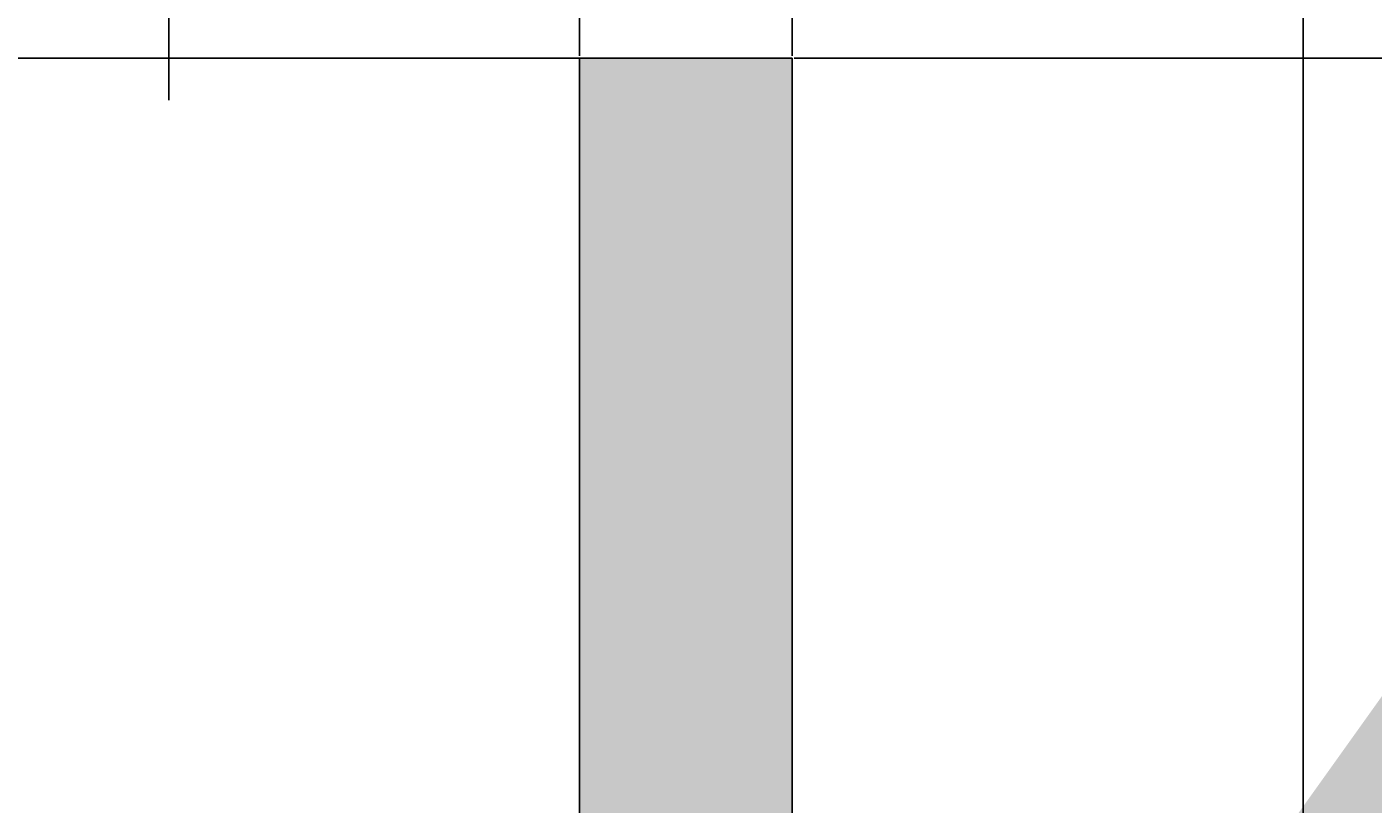
# Model space of a CAD drawing. Units: millimetres. Extents: x -22994 to 29398, y -19990 to 20176.
# Tile 112 of 135: x 166 to 204, y 155 to 177. Entities that reach past the tile are written whole.
import ezdxf

# ---------------------------------------------------------------- set-up
doc = ezdxf.new("R2010")
doc.units = ezdxf.units.MM
doc.header["$MEASUREMENT"] = 0
for name, color, linetype, lineweight in [('M-ANNO-SYMB', 7, 'Continuous', 25), ('M-DIMS', 2, 'Continuous', 18), ('M-EQPM', 7, 'Continuous', 25), ('M-EQPM-PATT', 7, 'Continuous', 18)]:
    doc.layers.add(name, color=color, linetype=linetype, lineweight=lineweight)
doc.styles.get("Standard").update_dxf_attribs({"font": 'arial.ttf'})
doc.dimstyles.get("Standard").update_dxf_attribs({"dimtxt": 0.18, "dimasz": 10000, "dimexe": 0.18, "dimexo": 0.0625, "dimgap": 0.09, "dimtad": 0, "dimtih": 1, "dimtoh": 1, "dimdec": 0, "dimzin": 0, "dimdsep": 46, "dimtxsty": 'Standard', "dimcen": 0.09, "dimadec": 0, "dimazin": 0, "dimtfac": 1, "dimtdec": 0, "dimtofl": 0, "dimtmove": 0, "dimatfit": 3, "dimfxl": 1, "dimtolj": 1, "dimtzin": 0, "dimlwd": 30, "dimarcsym": 0})

# ---------------------------------------------------------------- blocks, each defined once
blk = doc.blocks.new('*D2')
at = {"layer": 'Defpoints', "color": 0, "transparency": 16777216}
for p in [(6.677, 10.271), (290.852, 10.271), (290.852, -5.079)]:
    blk.add_point(p, dxfattribs=at)
at = {"layer": 'M-DIMS', "color": 0, "lineweight": -2, "transparency": 16777216}
for p, q in [((6.677, 10.209), (6.677, -5.259)), ((290.852, 10.209), (290.852, -5.259))]:
    blk.add_line(p, q, dxfattribs=at)
at = {"layer": 'M-DIMS', "color": 0, "lineweight": 30, "transparency": 16777216}
for p, q in [((-9993.323, -5.079), (-19993.323, -5.079)), ((10290.852, -5.079), (20290.852, -5.079))]:
    blk.add_line(p, q, dxfattribs=at)
at = {"layer": 'M-DIMS', "color": 0, "transparency": 16777216}
for points in [[(-9993.323, 1661.588), (-9993.323, -1671.745), (6.677, -5.079)], [(10290.852, 1661.588), (10290.852, -1671.745), (290.852, -5.079)]]:
    blk.add_solid(points, dxfattribs=at)
at = {"layer": 'M-DIMS', "color": 0, "transparency": 16777216, "insert": (148.765, -5.079), "char_height": 0.18, "attachment_point": 5}
blk.add_mtext('\\A1;284.2', dxfattribs=at)
blk = doc.blocks.new('*D3')
at = {"layer": 'Defpoints', "color": 0, "transparency": 16777216}
for p in [(110.265, 204.165), (110.265, 176.366), (95.833, 127.967)]:
    blk.add_point(p, dxfattribs=at)
at = {"layer": 'M-DIMS', "color": 0, "lineweight": 30, "transparency": 16777216}
for p, q in [((-9904.167, 204.165), (-19904.167, 204.165)), ((10110.265, 204.165), (20110.265, 204.165))]:
    blk.add_line(p, q, dxfattribs=at)
at = {"layer": 'M-DIMS', "color": 0, "lineweight": -2, "transparency": 16777216}
for p, q in [((95.833, 128.03), (95.833, 204.345)), ((110.265, 176.429), (110.265, 204.345))]:
    blk.add_line(p, q, dxfattribs=at)
at = {"layer": 'M-DIMS', "color": 0, "transparency": 16777216}
for points in [[(-9904.167, 1870.832), (-9904.167, -1462.501), (95.833, 204.165)], [(10110.265, 1870.832), (10110.265, -1462.501), (110.265, 204.165)]]:
    blk.add_solid(points, dxfattribs=at)
at = {"layer": 'M-DIMS', "color": 0, "transparency": 16777216, "insert": (103.049, 204.165), "char_height": 0.18, "attachment_point": 5}
blk.add_mtext('\\A1;14.432', dxfattribs=at)
blk = doc.blocks.new('*D4')
at = {"layer": 'Defpoints', "color": 0, "transparency": 16777216}
for p in [(116.265, 204.165), (110.265, 176.366), (116.265, 176.366)]:
    blk.add_point(p, dxfattribs=at)
at = {"layer": 'M-DIMS', "color": 0, "lineweight": 30, "transparency": 16777216}
for p, q in [((-9889.735, 204.165), (-19889.735, 204.165)), ((10116.265, 204.165), (20116.265, 204.165))]:
    blk.add_line(p, q, dxfattribs=at)
at = {"layer": 'M-DIMS', "color": 0, "lineweight": -2, "transparency": 16777216}
for p, q in [((110.265, 176.429), (110.265, 204.345)), ((116.265, 176.429), (116.265, 204.345))]:
    blk.add_line(p, q, dxfattribs=at)
at = {"layer": 'M-DIMS', "color": 0, "transparency": 16777216}
for points in [[(-9889.735, 1870.832), (-9889.735, -1462.501), (110.265, 204.165)], [(10116.265, 1870.832), (10116.265, -1462.501), (116.265, 204.165)]]:
    blk.add_solid(points, dxfattribs=at)
at = {"layer": 'M-DIMS', "color": 0, "transparency": 16777216, "insert": (113.265, 204.165), "char_height": 0.18, "attachment_point": 5}
blk.add_mtext('\\A1;6', dxfattribs=at)
blk = doc.blocks.new('*D5')
at = {"layer": 'Defpoints', "color": 0, "transparency": 16777216}
for p in [(181.265, 204.165), (116.265, 176.366), (181.265, 176.366)]:
    blk.add_point(p, dxfattribs=at)
at = {"layer": 'M-DIMS', "color": 0, "lineweight": 30, "transparency": 16777216}
for p, q in [((-9883.735, 204.165), (-19883.735, 204.165)), ((10181.265, 204.165), (20181.265, 204.165))]:
    blk.add_line(p, q, dxfattribs=at)
at = {"layer": 'M-DIMS', "color": 0, "lineweight": -2, "transparency": 16777216}
for p, q in [((116.265, 176.429), (116.265, 204.345)), ((181.265, 176.429), (181.265, 204.345))]:
    blk.add_line(p, q, dxfattribs=at)
at = {"layer": 'M-DIMS', "color": 0, "transparency": 16777216}
for points in [[(-9883.735, 1870.832), (-9883.735, -1462.501), (116.265, 204.165)], [(10181.265, 1870.832), (10181.265, -1462.501), (181.265, 204.165)]]:
    blk.add_solid(points, dxfattribs=at)
at = {"layer": 'M-DIMS', "color": 0, "transparency": 16777216, "insert": (148.765, 204.165), "char_height": 0.18, "attachment_point": 5}
blk.add_mtext('\\A1;65', dxfattribs=at)
blk = doc.blocks.new('*D6')
at = {"layer": 'Defpoints', "color": 0, "transparency": 16777216}
for p in [(187.265, 204.165), (181.265, 176.366), (187.265, 176.366)]:
    blk.add_point(p, dxfattribs=at)
at = {"layer": 'M-DIMS', "color": 0, "lineweight": 30, "transparency": 16777216}
for p, q in [((-9818.735, 204.165), (-19818.735, 204.165)), ((10187.265, 204.165), (20187.265, 204.165))]:
    blk.add_line(p, q, dxfattribs=at)
at = {"layer": 'M-DIMS', "color": 0, "lineweight": -2, "transparency": 16777216}
for p, q in [((181.265, 176.429), (181.265, 204.345)), ((187.265, 176.429), (187.265, 204.345))]:
    blk.add_line(p, q, dxfattribs=at)
at = {"layer": 'M-DIMS', "color": 0, "transparency": 16777216}
for points in [[(-9818.735, 1870.832), (-9818.735, -1462.501), (181.265, 204.165)], [(10187.265, 1870.832), (10187.265, -1462.501), (187.265, 204.165)]]:
    blk.add_solid(points, dxfattribs=at)
at = {"layer": 'M-DIMS', "color": 0, "transparency": 16777216, "insert": (184.265, 204.165), "char_height": 0.18, "attachment_point": 5}
blk.add_mtext('\\A1;6', dxfattribs=at)
blk = doc.blocks.new('*D7')
at = {"layer": 'Defpoints', "color": 0, "transparency": 16777216}
for p in [(201.697, 204.165), (187.265, 176.366), (201.697, 127.967)]:
    blk.add_point(p, dxfattribs=at)
at = {"layer": 'M-DIMS', "color": 0, "lineweight": 30, "transparency": 16777216}
for p, q in [((-9812.735, 204.165), (-19812.735, 204.165)), ((10201.697, 204.165), (20201.697, 204.165))]:
    blk.add_line(p, q, dxfattribs=at)
at = {"layer": 'M-DIMS', "color": 0, "lineweight": -2, "transparency": 16777216}
for p, q in [((187.265, 176.429), (187.265, 204.345)), ((201.697, 128.03), (201.697, 204.345))]:
    blk.add_line(p, q, dxfattribs=at)
at = {"layer": 'M-DIMS', "color": 0, "transparency": 16777216}
for points in [[(-9812.735, 1870.832), (-9812.735, -1462.501), (187.265, 204.165)], [(10201.697, 1870.832), (10201.697, -1462.501), (201.697, 204.165)]]:
    blk.add_solid(points, dxfattribs=at)
at = {"layer": 'M-DIMS', "color": 0, "transparency": 16777216, "insert": (194.481, 204.165), "char_height": 0.18, "attachment_point": 5}
blk.add_mtext('\\A1;14.432', dxfattribs=at)
blk = doc.blocks.new('*D8')
at = {"layer": 'Defpoints', "color": 0, "transparency": 16777216}
for p in [(227.648, 204.165), (227.648, 146.73), (201.697, 127.967)]:
    blk.add_point(p, dxfattribs=at)
at = {"layer": 'M-DIMS', "color": 0, "lineweight": 30, "transparency": 16777216}
for p, q in [((-9798.303, 204.165), (-19798.303, 204.165)), ((10227.648, 204.165), (20227.648, 204.165))]:
    blk.add_line(p, q, dxfattribs=at)
at = {"layer": 'M-DIMS', "color": 0, "lineweight": -2, "transparency": 16777216}
for p, q in [((201.697, 128.03), (201.697, 204.345)), ((227.648, 146.792), (227.648, 204.345))]:
    blk.add_line(p, q, dxfattribs=at)
at = {"layer": 'M-DIMS', "color": 0, "transparency": 16777216}
for points in [[(-9798.303, 1870.832), (-9798.303, -1462.501), (201.697, 204.165)], [(10227.648, 1870.832), (10227.648, -1462.501), (227.648, 204.165)]]:
    blk.add_solid(points, dxfattribs=at)
at = {"layer": 'M-DIMS', "color": 0, "transparency": 16777216, "insert": (214.673, 204.165), "char_height": 0.18, "attachment_point": 5}
blk.add_mtext('\\A1;25.95', dxfattribs=at)
blk = doc.blocks.new('*D9')
at = {"layer": 'Defpoints', "color": 0, "transparency": 16777216}
for p in [(187.265, 176.366), (306.202, 176.366), (290.852, 10.271)]:
    blk.add_point(p, dxfattribs=at)
at = {"layer": 'M-DIMS', "color": 0, "lineweight": 30, "transparency": 16777216}
for p, q in [((306.202, 10176.366), (306.202, 20176.366)), ((306.202, -9989.729), (306.202, -19989.729))]:
    blk.add_line(p, q, dxfattribs=at)
at = {"layer": 'M-DIMS', "color": 0, "lineweight": -2, "transparency": 16777216}
for p, q in [((187.327, 176.366), (306.382, 176.366)), ((290.915, 10.271), (306.382, 10.271))]:
    blk.add_line(p, q, dxfattribs=at)
at = {"layer": 'M-DIMS', "color": 0, "transparency": 16777216}
for points in [[(-1360.465, 10176.366), (1972.869, 10176.366), (306.202, 176.366)], [(-1360.465, -9989.729), (1972.869, -9989.729), (306.202, 10.271)]]:
    blk.add_solid(points, dxfattribs=at)
at = {"layer": 'M-DIMS', "color": 0, "transparency": 16777216, "insert": (306.202, 93.319), "char_height": 0.18, "attachment_point": 5}
blk.add_mtext('\\A1;166.1', dxfattribs=at)
blk = doc.blocks.new('*D10')
at = {"layer": 'Defpoints', "color": 0, "transparency": 16777216}
for p in [(125.65, 136.071), (133.346, 136.071), (133.346, -5.079)]:
    blk.add_point(p, dxfattribs=at)
at = {"layer": 'M-DIMS', "color": 0, "lineweight": -2, "transparency": 16777216}
for p, q in [((125.65, 136.009), (125.65, -5.259)), ((133.346, 136.009), (133.346, -5.259))]:
    blk.add_line(p, q, dxfattribs=at)
at = {"layer": 'M-DIMS', "color": 0, "lineweight": 30, "transparency": 16777216}
for p, q in [((-9874.35, -5.079), (-19874.35, -5.079)), ((10133.346, -5.079), (20133.346, -5.079))]:
    blk.add_line(p, q, dxfattribs=at)
at = {"layer": 'M-DIMS', "color": 0, "transparency": 16777216}
for points in [[(-9874.35, 1661.588), (-9874.35, -1671.745), (125.65, -5.079)], [(10133.346, 1661.588), (10133.346, -1671.745), (133.346, -5.079)]]:
    blk.add_solid(points, dxfattribs=at)
at = {"layer": 'M-DIMS', "color": 0, "transparency": 16777216, "insert": (129.498, -5.079), "char_height": 0.18, "attachment_point": 5}
blk.add_mtext('\\A1;7.696', dxfattribs=at)
blk = doc.blocks.new('*D11')
at = {"layer": 'Defpoints', "color": 0, "transparency": 16777216}
for p in [(133.346, 136.071), (135.65, 136.071), (135.65, -5.079)]:
    blk.add_point(p, dxfattribs=at)
at = {"layer": 'M-DIMS', "color": 0, "lineweight": -2, "transparency": 16777216}
for p, q in [((133.346, 136.009), (133.346, -5.259)), ((135.65, 136.009), (135.65, -5.259))]:
    blk.add_line(p, q, dxfattribs=at)
at = {"layer": 'M-DIMS', "color": 0, "lineweight": 30, "transparency": 16777216}
for p, q in [((-9866.654, -5.079), (-19866.654, -5.079)), ((10135.65, -5.079), (20135.65, -5.079))]:
    blk.add_line(p, q, dxfattribs=at)
at = {"layer": 'M-DIMS', "color": 0, "transparency": 16777216}
for points in [[(-9866.654, 1661.588), (-9866.654, -1671.745), (133.346, -5.079)], [(10135.65, 1661.588), (10135.65, -1671.745), (135.65, -5.079)]]:
    blk.add_solid(points, dxfattribs=at)
at = {"layer": 'M-DIMS', "color": 0, "transparency": 16777216, "insert": (134.498, -5.079), "char_height": 0.18, "attachment_point": 5}
blk.add_mtext('\\A1;2.304', dxfattribs=at)
blk = doc.blocks.new('*D12')
at = {"layer": 'Defpoints', "color": 0, "transparency": 16777216}
for p in [(135.65, 136.071), (145.65, 136.071), (145.65, -5.079)]:
    blk.add_point(p, dxfattribs=at)
at = {"layer": 'M-DIMS', "color": 0, "lineweight": -2, "transparency": 16777216}
for p, q in [((135.65, 136.009), (135.65, -5.259)), ((145.65, 136.009), (145.65, -5.259))]:
    blk.add_line(p, q, dxfattribs=at)
at = {"layer": 'M-DIMS', "color": 0, "lineweight": 30, "transparency": 16777216}
for p, q in [((-9864.35, -5.079), (-19864.35, -5.079)), ((10145.65, -5.079), (20145.65, -5.079))]:
    blk.add_line(p, q, dxfattribs=at)
at = {"layer": 'M-DIMS', "color": 0, "transparency": 16777216}
for points in [[(-9864.35, 1661.588), (-9864.35, -1671.745), (135.65, -5.079)], [(10145.65, 1661.588), (10145.65, -1671.745), (145.65, -5.079)]]:
    blk.add_solid(points, dxfattribs=at)
at = {"layer": 'M-DIMS', "color": 0, "transparency": 16777216, "insert": (140.65, -5.079), "char_height": 0.18, "attachment_point": 5}
blk.add_mtext('\\A1;10', dxfattribs=at)
blk = doc.blocks.new('*D13')
at = {"layer": 'Defpoints', "color": 0, "transparency": 16777216}
for p in [(145.65, 136.071), (155.65, 136.071), (155.65, -5.079)]:
    blk.add_point(p, dxfattribs=at)
at = {"layer": 'M-DIMS', "color": 0, "lineweight": -2, "transparency": 16777216}
for p, q in [((145.65, 136.009), (145.65, -5.259)), ((155.65, 136.009), (155.65, -5.259))]:
    blk.add_line(p, q, dxfattribs=at)
at = {"layer": 'M-DIMS', "color": 0, "lineweight": 30, "transparency": 16777216}
for p, q in [((-9854.35, -5.079), (-19854.35, -5.079)), ((10155.65, -5.079), (20155.65, -5.079))]:
    blk.add_line(p, q, dxfattribs=at)
at = {"layer": 'M-DIMS', "color": 0, "transparency": 16777216}
for points in [[(-9854.35, 1661.588), (-9854.35, -1671.745), (145.65, -5.079)], [(10155.65, 1661.588), (10155.65, -1671.745), (155.65, -5.079)]]:
    blk.add_solid(points, dxfattribs=at)
at = {"layer": 'M-DIMS', "color": 0, "transparency": 16777216, "insert": (150.65, -5.079), "char_height": 0.18, "attachment_point": 5}
blk.add_mtext('\\A1;10', dxfattribs=at)
blk = doc.blocks.new('*D14')
at = {"layer": 'Defpoints', "color": 0, "transparency": 16777216}
for p in [(155.65, 136.071), (165.65, 136.071), (165.65, -5.079)]:
    blk.add_point(p, dxfattribs=at)
at = {"layer": 'M-DIMS', "color": 0, "lineweight": -2, "transparency": 16777216}
for p, q in [((155.65, 136.009), (155.65, -5.259)), ((165.65, 136.009), (165.65, -5.259))]:
    blk.add_line(p, q, dxfattribs=at)
at = {"layer": 'M-DIMS', "color": 0, "lineweight": 30, "transparency": 16777216}
for p, q in [((-9844.35, -5.079), (-19844.35, -5.079)), ((10165.65, -5.079), (20165.65, -5.079))]:
    blk.add_line(p, q, dxfattribs=at)
at = {"layer": 'M-DIMS', "color": 0, "transparency": 16777216}
for points in [[(-9844.35, 1661.588), (-9844.35, -1671.745), (155.65, -5.079)], [(10165.65, 1661.588), (10165.65, -1671.745), (165.65, -5.079)]]:
    blk.add_solid(points, dxfattribs=at)
at = {"layer": 'M-DIMS', "color": 0, "transparency": 16777216, "insert": (160.65, -5.079), "char_height": 0.18, "attachment_point": 5}
blk.add_mtext('\\A1;10', dxfattribs=at)
blk = doc.blocks.new('*D15')
at = {"layer": 'Defpoints', "color": 0, "transparency": 16777216}
for p in [(173.346, 154.788), (173.346, 136.071), (306.202, 136.071)]:
    blk.add_point(p, dxfattribs=at)
at = {"layer": 'M-DIMS', "color": 0, "lineweight": 30, "transparency": 16777216}
for p, q in [((306.202, 10154.788), (306.202, 20154.788)), ((306.202, -9863.929), (306.202, -19863.929))]:
    blk.add_line(p, q, dxfattribs=at)
at = {"layer": 'M-DIMS', "color": 0, "lineweight": -2, "transparency": 16777216}
for p, q in [((173.408, 154.788), (306.382, 154.788)), ((173.408, 136.071), (306.382, 136.071))]:
    blk.add_line(p, q, dxfattribs=at)
at = {"layer": 'M-DIMS', "color": 0, "transparency": 16777216}
for points in [[(-1360.465, 10154.788), (1972.869, 10154.788), (306.202, 154.788)], [(-1360.465, -9863.929), (1972.869, -9863.929), (306.202, 136.071)]]:
    blk.add_solid(points, dxfattribs=at)
at = {"layer": 'M-DIMS', "color": 0, "transparency": 16777216, "insert": (306.202, 145.43), "char_height": 0.18, "attachment_point": 5}
blk.add_mtext('\\A1;18.717', dxfattribs=at)
blk = doc.blocks.new('*D16')
at = {"layer": 'Defpoints', "color": 0, "transparency": 16777216}
for p in [(120.17, 204.165), (110.466, 48.035), (120.17, 48.035)]:
    blk.add_point(p, dxfattribs=at)
at = {"layer": 'M-DIMS', "color": 0, "lineweight": 30, "transparency": 16777216}
for p, q in [((-9889.534, 204.165), (-19889.534, 204.165)), ((10120.17, 204.165), (20120.17, 204.165))]:
    blk.add_line(p, q, dxfattribs=at)
at = {"layer": 'M-DIMS', "color": 0, "lineweight": -2, "transparency": 16777216}
for p, q in [((110.466, 48.097), (110.466, 204.345)), ((120.17, 48.097), (120.17, 204.345))]:
    blk.add_line(p, q, dxfattribs=at)
at = {"layer": 'M-DIMS', "color": 0, "transparency": 16777216}
for points in [[(-9889.534, 1870.832), (-9889.534, -1462.501), (110.466, 204.165)], [(10120.17, 1870.832), (10120.17, -1462.501), (120.17, 204.165)]]:
    blk.add_solid(points, dxfattribs=at)
at = {"layer": 'M-DIMS', "color": 0, "transparency": 16777216, "insert": (115.318, 204.165), "char_height": 0.18, "attachment_point": 5}
blk.add_mtext('\\A1;9.704', dxfattribs=at)
blk = doc.blocks.new('*D17')
at = {"layer": 'Defpoints', "color": 0, "transparency": 16777216}
for p in [(126.17, 204.165), (120.17, 48.035), (126.17, 48.035)]:
    blk.add_point(p, dxfattribs=at)
at = {"layer": 'M-DIMS', "color": 0, "lineweight": 30, "transparency": 16777216}
for p, q in [((-9879.83, 204.165), (-19879.83, 204.165)), ((10126.17, 204.165), (20126.17, 204.165))]:
    blk.add_line(p, q, dxfattribs=at)
at = {"layer": 'M-DIMS', "color": 0, "lineweight": -2, "transparency": 16777216}
for p, q in [((120.17, 48.097), (120.17, 204.345)), ((126.17, 48.097), (126.17, 204.345))]:
    blk.add_line(p, q, dxfattribs=at)
at = {"layer": 'M-DIMS', "color": 0, "transparency": 16777216}
for points in [[(-9879.83, 1870.832), (-9879.83, -1462.501), (120.17, 204.165)], [(10126.17, 1870.832), (10126.17, -1462.501), (126.17, 204.165)]]:
    blk.add_solid(points, dxfattribs=at)
at = {"layer": 'M-DIMS', "color": 0, "transparency": 16777216, "insert": (123.17, 204.165), "char_height": 0.18, "attachment_point": 5}
blk.add_mtext('\\A1;6', dxfattribs=at)
blk = doc.blocks.new('*D18')
at = {"layer": 'Defpoints', "color": 0, "transparency": 16777216}
for p in [(132.17, 204.165), (126.17, 48.035), (132.17, 48.035)]:
    blk.add_point(p, dxfattribs=at)
at = {"layer": 'M-DIMS', "color": 0, "lineweight": 30, "transparency": 16777216}
for p, q in [((-9873.83, 204.165), (-19873.83, 204.165)), ((10132.17, 204.165), (20132.17, 204.165))]:
    blk.add_line(p, q, dxfattribs=at)
at = {"layer": 'M-DIMS', "color": 0, "lineweight": -2, "transparency": 16777216}
for p, q in [((126.17, 48.097), (126.17, 204.345)), ((132.17, 48.097), (132.17, 204.345))]:
    blk.add_line(p, q, dxfattribs=at)
at = {"layer": 'M-DIMS', "color": 0, "transparency": 16777216}
for points in [[(-9873.83, 1870.832), (-9873.83, -1462.501), (126.17, 204.165)], [(10132.17, 1870.832), (10132.17, -1462.501), (132.17, 204.165)]]:
    blk.add_solid(points, dxfattribs=at)
at = {"layer": 'M-DIMS', "color": 0, "transparency": 16777216, "insert": (129.17, 204.165), "char_height": 0.18, "attachment_point": 5}
blk.add_mtext('\\A1;6', dxfattribs=at)
blk = doc.blocks.new('*D19')
at = {"layer": 'Defpoints', "color": 0, "transparency": 16777216}
for p in [(138.17, 204.165), (132.17, 48.035), (138.17, 48.035)]:
    blk.add_point(p, dxfattribs=at)
at = {"layer": 'M-DIMS', "color": 0, "lineweight": 30, "transparency": 16777216}
for p, q in [((-9867.83, 204.165), (-19867.83, 204.165)), ((10138.17, 204.165), (20138.17, 204.165))]:
    blk.add_line(p, q, dxfattribs=at)
at = {"layer": 'M-DIMS', "color": 0, "lineweight": -2, "transparency": 16777216}
for p, q in [((132.17, 48.097), (132.17, 204.345)), ((138.17, 48.097), (138.17, 204.345))]:
    blk.add_line(p, q, dxfattribs=at)
at = {"layer": 'M-DIMS', "color": 0, "transparency": 16777216}
for points in [[(-9867.83, 1870.832), (-9867.83, -1462.501), (132.17, 204.165)], [(10138.17, 1870.832), (10138.17, -1462.501), (138.17, 204.165)]]:
    blk.add_solid(points, dxfattribs=at)
at = {"layer": 'M-DIMS', "color": 0, "transparency": 16777216, "insert": (135.17, 204.165), "char_height": 0.18, "attachment_point": 5}
blk.add_mtext('\\A1;6', dxfattribs=at)
blk = doc.blocks.new('*D20')
at = {"layer": 'Defpoints', "color": 0, "transparency": 16777216}
for p in [(144.17, 204.165), (138.17, 48.035), (144.17, 48.035)]:
    blk.add_point(p, dxfattribs=at)
at = {"layer": 'M-DIMS', "color": 0, "lineweight": 30, "transparency": 16777216}
for p, q in [((-9861.83, 204.165), (-19861.83, 204.165)), ((10144.17, 204.165), (20144.17, 204.165))]:
    blk.add_line(p, q, dxfattribs=at)
at = {"layer": 'M-DIMS', "color": 0, "lineweight": -2, "transparency": 16777216}
for p, q in [((138.17, 48.097), (138.17, 204.345)), ((144.17, 48.097), (144.17, 204.345))]:
    blk.add_line(p, q, dxfattribs=at)
at = {"layer": 'M-DIMS', "color": 0, "transparency": 16777216}
for points in [[(-9861.83, 1870.832), (-9861.83, -1462.501), (138.17, 204.165)], [(10144.17, 1870.832), (10144.17, -1462.501), (144.17, 204.165)]]:
    blk.add_solid(points, dxfattribs=at)
at = {"layer": 'M-DIMS', "color": 0, "transparency": 16777216, "insert": (141.17, 204.165), "char_height": 0.18, "attachment_point": 5}
blk.add_mtext('\\A1;6', dxfattribs=at)
blk = doc.blocks.new('*D21')
at = {"layer": 'Defpoints', "color": 0, "transparency": 16777216}
for p in [(149.116, 204.165), (144.17, 48.035), (149.116, 48.035)]:
    blk.add_point(p, dxfattribs=at)
at = {"layer": 'M-DIMS', "color": 0, "lineweight": 30, "transparency": 16777216}
for p, q in [((-9855.83, 204.165), (-19855.83, 204.165)), ((10149.116, 204.165), (20149.116, 204.165))]:
    blk.add_line(p, q, dxfattribs=at)
at = {"layer": 'M-DIMS', "color": 0, "lineweight": -2, "transparency": 16777216}
for p, q in [((144.17, 48.097), (144.17, 204.345)), ((149.116, 48.097), (149.116, 204.345))]:
    blk.add_line(p, q, dxfattribs=at)
at = {"layer": 'M-DIMS', "color": 0, "transparency": 16777216}
for points in [[(-9855.83, 1870.832), (-9855.83, -1462.501), (144.17, 204.165)], [(10149.116, 1870.832), (10149.116, -1462.501), (149.116, 204.165)]]:
    blk.add_solid(points, dxfattribs=at)
at = {"layer": 'M-DIMS', "color": 0, "transparency": 16777216, "insert": (146.643, 204.165), "char_height": 0.18, "attachment_point": 5}
blk.add_mtext('\\A1;4.945', dxfattribs=at)
blk = doc.blocks.new('*D22')
at = {"layer": 'Defpoints', "color": 0, "transparency": 16777216}
for p in [(149.116, 30.99), (155.116, 30.99), (155.116, -5.079)]:
    blk.add_point(p, dxfattribs=at)
at = {"layer": 'M-DIMS', "color": 0, "lineweight": -2, "transparency": 16777216}
for p, q in [((149.116, 30.927), (149.116, -5.259)), ((155.116, 30.927), (155.116, -5.259))]:
    blk.add_line(p, q, dxfattribs=at)
at = {"layer": 'M-DIMS', "color": 0, "lineweight": 30, "transparency": 16777216}
for p, q in [((-9850.884, -5.079), (-19850.884, -5.079)), ((10155.116, -5.079), (20155.116, -5.079))]:
    blk.add_line(p, q, dxfattribs=at)
at = {"layer": 'M-DIMS', "color": 0, "transparency": 16777216}
for points in [[(-9850.884, 1661.588), (-9850.884, -1671.745), (149.116, -5.079)], [(10155.116, 1661.588), (10155.116, -1671.745), (155.116, -5.079)]]:
    blk.add_solid(points, dxfattribs=at)
at = {"layer": 'M-DIMS', "color": 0, "transparency": 16777216, "insert": (152.116, -5.079), "char_height": 0.18, "attachment_point": 5}
blk.add_mtext('\\A1;6', dxfattribs=at)
blk = doc.blocks.new('*D23')
at = {"layer": 'Defpoints', "color": 0, "transparency": 16777216}
for p in [(155.116, 30.99), (161.116, 30.99), (161.116, -5.079)]:
    blk.add_point(p, dxfattribs=at)
at = {"layer": 'M-DIMS', "color": 0, "lineweight": -2, "transparency": 16777216}
for p, q in [((155.116, 30.927), (155.116, -5.259)), ((161.116, 30.927), (161.116, -5.259))]:
    blk.add_line(p, q, dxfattribs=at)
at = {"layer": 'M-DIMS', "color": 0, "lineweight": 30, "transparency": 16777216}
for p, q in [((-9844.884, -5.079), (-19844.884, -5.079)), ((10161.116, -5.079), (20161.116, -5.079))]:
    blk.add_line(p, q, dxfattribs=at)
at = {"layer": 'M-DIMS', "color": 0, "transparency": 16777216}
for points in [[(-9844.884, 1661.588), (-9844.884, -1671.745), (155.116, -5.079)], [(10161.116, 1661.588), (10161.116, -1671.745), (161.116, -5.079)]]:
    blk.add_solid(points, dxfattribs=at)
at = {"layer": 'M-DIMS', "color": 0, "transparency": 16777216, "insert": (158.116, -5.079), "char_height": 0.18, "attachment_point": 5}
blk.add_mtext('\\A1;6', dxfattribs=at)
blk = doc.blocks.new('*D24')
at = {"layer": 'Defpoints', "color": 0, "transparency": 16777216}
for p in [(161.116, 30.99), (166.439, 30.99), (166.439, -5.079)]:
    blk.add_point(p, dxfattribs=at)
at = {"layer": 'M-DIMS', "color": 0, "lineweight": -2, "transparency": 16777216}
for p, q in [((161.116, 30.927), (161.116, -5.259)), ((166.439, 30.927), (166.439, -5.259))]:
    blk.add_line(p, q, dxfattribs=at)
at = {"layer": 'M-DIMS', "color": 0, "lineweight": 30, "transparency": 16777216}
for p, q in [((-9838.884, -5.079), (-19838.884, -5.079)), ((10166.439, -5.079), (20166.439, -5.079))]:
    blk.add_line(p, q, dxfattribs=at)
at = {"layer": 'M-DIMS', "color": 0, "transparency": 16777216}
for points in [[(-9838.884, 1661.588), (-9838.884, -1671.745), (161.116, -5.079)], [(10166.439, 1661.588), (10166.439, -1671.745), (166.439, -5.079)]]:
    blk.add_solid(points, dxfattribs=at)
at = {"layer": 'M-DIMS', "color": 0, "transparency": 16777216, "insert": (163.777, -5.079), "char_height": 0.18, "attachment_point": 5}
blk.add_mtext('\\A1;5.323', dxfattribs=at)
blk = doc.blocks.new('*D25')
at = {"layer": 'Defpoints', "color": 0, "transparency": 16777216}
for p in [(166.439, 30.99), (172.439, 30.99), (172.439, -5.079)]:
    blk.add_point(p, dxfattribs=at)
at = {"layer": 'M-DIMS', "color": 0, "lineweight": -2, "transparency": 16777216}
for p, q in [((166.439, 30.927), (166.439, -5.259)), ((172.439, 30.927), (172.439, -5.259))]:
    blk.add_line(p, q, dxfattribs=at)
at = {"layer": 'M-DIMS', "color": 0, "lineweight": 30, "transparency": 16777216}
for p, q in [((-9833.561, -5.079), (-19833.561, -5.079)), ((10172.439, -5.079), (20172.439, -5.079))]:
    blk.add_line(p, q, dxfattribs=at)
at = {"layer": 'M-DIMS', "color": 0, "transparency": 16777216}
for points in [[(-9833.561, 1661.588), (-9833.561, -1671.745), (166.439, -5.079)], [(10172.439, 1661.588), (10172.439, -1671.745), (172.439, -5.079)]]:
    blk.add_solid(points, dxfattribs=at)
at = {"layer": 'M-DIMS', "color": 0, "transparency": 16777216, "insert": (169.439, -5.079), "char_height": 0.18, "attachment_point": 5}
blk.add_mtext('\\A1;6', dxfattribs=at)
blk = doc.blocks.new('*D26')
at = {"layer": 'Defpoints', "color": 0, "transparency": 16777216}
for p in [(172.439, 30.99), (178.439, 30.99), (178.439, -5.079)]:
    blk.add_point(p, dxfattribs=at)
at = {"layer": 'M-DIMS', "color": 0, "lineweight": -2, "transparency": 16777216}
for p, q in [((172.439, 30.927), (172.439, -5.259)), ((178.439, 30.927), (178.439, -5.259))]:
    blk.add_line(p, q, dxfattribs=at)
at = {"layer": 'M-DIMS', "color": 0, "lineweight": 30, "transparency": 16777216}
for p, q in [((-9827.561, -5.079), (-19827.561, -5.079)), ((10178.439, -5.079), (20178.439, -5.079))]:
    blk.add_line(p, q, dxfattribs=at)
at = {"layer": 'M-DIMS', "color": 0, "transparency": 16777216}
for points in [[(-9827.561, 1661.588), (-9827.561, -1671.745), (172.439, -5.079)], [(10178.439, 1661.588), (10178.439, -1671.745), (178.439, -5.079)]]:
    blk.add_solid(points, dxfattribs=at)
at = {"layer": 'M-DIMS', "color": 0, "transparency": 16777216, "insert": (175.439, -5.079), "char_height": 0.18, "attachment_point": 5}
blk.add_mtext('\\A1;6', dxfattribs=at)
blk = doc.blocks.new('*D27')
at = {"layer": 'Defpoints', "color": 0, "transparency": 16777216}
for p in [(178.439, 30.99), (188.117, 30.99), (188.117, -5.079)]:
    blk.add_point(p, dxfattribs=at)
at = {"layer": 'M-DIMS', "color": 0, "lineweight": -2, "transparency": 16777216}
for p, q in [((178.439, 30.927), (178.439, -5.259)), ((188.117, 30.927), (188.117, -5.259))]:
    blk.add_line(p, q, dxfattribs=at)
at = {"layer": 'M-DIMS', "color": 0, "lineweight": 30, "transparency": 16777216}
for p, q in [((-9821.561, -5.079), (-19821.561, -5.079)), ((10188.117, -5.079), (20188.117, -5.079))]:
    blk.add_line(p, q, dxfattribs=at)
at = {"layer": 'M-DIMS', "color": 0, "transparency": 16777216}
for points in [[(-9821.561, 1661.588), (-9821.561, -1671.745), (178.439, -5.079)], [(10188.117, 1661.588), (10188.117, -1671.745), (188.117, -5.079)]]:
    blk.add_solid(points, dxfattribs=at)
at = {"layer": 'M-DIMS', "color": 0, "transparency": 16777216, "insert": (183.278, -5.079), "char_height": 0.18, "attachment_point": 5}
blk.add_mtext('\\A1;9.679', dxfattribs=at)
blk = doc.blocks.new('*D28')
at = {"layer": 'Defpoints', "color": 0, "transparency": 16777216}
for p in [(188.117, 48.035), (306.202, 48.035), (188.117, 30.99)]:
    blk.add_point(p, dxfattribs=at)
at = {"layer": 'M-DIMS', "color": 0, "lineweight": 30, "transparency": 16777216}
for p, q in [((306.202, 10048.035), (306.202, 20048.035)), ((306.202, -9969.01), (306.202, -19969.01))]:
    blk.add_line(p, q, dxfattribs=at)
at = {"layer": 'M-DIMS', "color": 0, "lineweight": -2, "transparency": 16777216}
for p, q in [((188.18, 48.035), (306.382, 48.035)), ((188.18, 30.99), (306.382, 30.99))]:
    blk.add_line(p, q, dxfattribs=at)
at = {"layer": 'M-DIMS', "color": 0, "transparency": 16777216}
for points in [[(-1360.465, 10048.035), (1972.869, 10048.035), (306.202, 48.035)], [(-1360.465, -9969.01), (1972.869, -9969.01), (306.202, 30.99)]]:
    blk.add_solid(points, dxfattribs=at)
at = {"layer": 'M-DIMS', "color": 0, "transparency": 16777216, "insert": (306.202, 39.512), "char_height": 0.18, "attachment_point": 5}
blk.add_mtext('\\A1;17.045', dxfattribs=at)
blk = doc.blocks.new('*D29')
at = {"layer": 'Defpoints', "color": 0, "transparency": 16777216}
for p in [(36.801, 80.045), (64.03, 80.045)]:
    blk.add_point(p, dxfattribs=at)
at = {"layer": 'M-DIMS', "color": 0, "lineweight": -2, "transparency": 16777216}
for p, q in [((50.325, 80.045), (50.505, 80.045)), ((50.415, 79.955), (50.415, 80.135))]:
    blk.add_line(p, q, dxfattribs=at)
at = {"layer": 'M-DIMS', "color": 0, "lineweight": 30, "transparency": 16777216}
blk.add_line((20064.03, 80.03), (10064.03, 80.038), dxfattribs=at)
at = {"layer": 'M-DIMS', "color": 0, "transparency": 16777216}
blk.add_solid([(10064.031, 1746.704), (10064.028, -1586.629), (64.03, 80.045)], dxfattribs=at)
at = {"layer": 'M-DIMS', "color": 0, "transparency": 16777216, "insert": (20064.521, 80.03), "char_height": 0.18, "attachment_point": 5}
blk.add_mtext('\\A1;∅27.23', dxfattribs=at)
blk = doc.blocks.new('*D34')
at = {"layer": 'Defpoints', "color": 0, "transparency": 16777216}
for p in [(178.58, 122.895), (176.812, 121.128)]:
    blk.add_point(p, dxfattribs=at)
at = {"layer": 'M-DIMS', "color": 0, "lineweight": 30, "transparency": 16777216}
for p, q in [((14322.436, 14263.311), (7250.508, 7193.103)), ((24322.436, 14263.311), (14322.436, 14263.311))]:
    blk.add_line(p, q, dxfattribs=at)
at = {"layer": 'M-DIMS', "color": 0, "lineweight": -2, "transparency": 16777216}
for p, q in [((176.722, 121.128), (176.902, 121.128)), ((176.812, 121.038), (176.812, 121.218))]:
    blk.add_line(p, q, dxfattribs=at)
at = {"layer": 'M-DIMS', "color": 0, "transparency": 16777216}
blk.add_solid([(6072.14, 8371.758), (8428.876, 6014.448), (178.58, 122.895)], dxfattribs=at)
at = {"layer": 'M-DIMS', "color": 0, "transparency": 16777216, "insert": (24322.97, 14263.311), "char_height": 0.18, "attachment_point": 5}
blk.add_mtext('\\A1;6X R2.5', dxfattribs=at)
blk = doc.blocks.new('*D36')
at = {"layer": 'Defpoints', "color": 0, "transparency": 16777216}
for p in [(46.39, 31.303), (46.387, 26.593)]:
    blk.add_point(p, dxfattribs=at)
at = {"layer": 'M-DIMS', "color": 0, "lineweight": 30, "transparency": 16777216}
for p, q in [((57.15, 20031.301), (51.77, 10031.302)), ((10057.15, 20031.301), (57.15, 20031.301))]:
    blk.add_line(p, q, dxfattribs=at)
at = {"layer": 'M-DIMS', "color": 0, "lineweight": -2, "transparency": 16777216}
for p, q in [((46.299, 28.948), (46.479, 28.948)), ((46.389, 28.858), (46.389, 29.038))]:
    blk.add_line(p, q, dxfattribs=at)
at = {"layer": 'M-DIMS', "color": 0, "transparency": 16777216}
blk.add_solid([(-1614.896, 10032.199), (1718.436, 10030.405), (46.39, 31.303)], dxfattribs=at)
at = {"layer": 'M-DIMS', "color": 0, "transparency": 16777216, "insert": (10057.554, 20031.301), "char_height": 0.18, "attachment_point": 5}
blk.add_mtext('\\A1;∅4.71', dxfattribs=at)
blk = doc.blocks.new('*D37')
at = {"layer": 'Defpoints', "color": 0, "transparency": 16777216}
for p in [(54.834, 118.615), (59.494, 118.614)]:
    blk.add_point(p, dxfattribs=at)
at = {"layer": 'M-DIMS', "color": 0, "lineweight": -2, "transparency": 16777216}
for p, q in [((57.074, 118.614), (57.254, 118.614)), ((57.164, 118.524), (57.164, 118.704))]:
    blk.add_line(p, q, dxfattribs=at)
at = {"layer": 'M-DIMS', "color": 0, "lineweight": 30, "transparency": 16777216}
blk.add_line((20059.493, 116.253), (10059.494, 117.434), dxfattribs=at)
at = {"layer": 'M-DIMS', "color": 0, "transparency": 16777216}
blk.add_solid([(10059.69, 1784.1), (10059.297, -1549.233), (59.494, 118.614)], dxfattribs=at)
at = {"layer": 'M-DIMS', "color": 0, "transparency": 16777216, "insert": (20059.985, 116.253), "char_height": 0.18, "attachment_point": 5}
blk.add_mtext('\\A1;∅4.659', dxfattribs=at)

msp = doc.modelspace()

# ---------------------------------------------------------------- hatches: boundary and pattern name
at = {"layer": 'M-EQPM-PATT'}
h = msp.add_hatch(color=256, dxfattribs=at)
h.set_gradient(color1=(205, 32, 39), color2=(205, 32, 39), tint=1)
h.paths.add_polyline_path([(116.2647, 150.3662), (116.2647, 170.3662), (116.2647, 176.3662), (110.2647, 176.3662), (110.2647, 152.0276), (95.8327, 127.967), (95.8327, 16.6063), (201.6967, 16.6063), (201.6967, 127.967), (187.2647, 152.0276), (187.2647, 176.3662), (181.2647, 176.3662), (181.2647, 170.3662), (181.2647, 150.3662), (195.6967, 126.3055), (195.6967, 22.6063), (101.8327, 22.6063), (101.8327, 126.3055)])
h.paths.add_polyline_path([(185.2208, 88.6347), (101.8327, 88.6347), (101.8327, 87.6347), (182.8066, 87.6347), (178.7313, 83.5594), (195.6967, 83.5594), (195.6967, 84.5594), (181.1455, 84.5594)], flags=17)
h.paths.add_polyline_path([(95.8327, 88.6347), (60.9779, 88.6347, -0.0228552), (61.7178, 87.6347), (95.8327, 87.6347)])
h.paths.add_polyline_path([(215.6212, 86.5189), (215.6212, 80.5999), (220.5095, 83.5594)])
h.paths.add_polyline_path([(215.6212, 84.5594), (201.6967, 84.5594), (201.6967, 83.5594), (215.6212, 83.5594)])
h.paths.add_polyline_path([(225.3978, 86.5189), (220.5095, 83.5594), (225.3978, 80.5999)])
h.paths.add_polyline_path([(231.6256, 84.5594), (225.3978, 84.5594), (225.3978, 83.5594), (231.6256, 83.5594)])

# ---------------------------------------------------------------- linework, layer by layer
at = {"layer": 'M-ANNO-SYMB'}
msp.add_line((169.6701, 184.2067), (169.6701, 175.1778), dxfattribs=at)
at = {"layer": 'M-EQPM'}
msp.add_line((181.2647, 170.3662), (181.2647, 176.3662), dxfattribs=at)
msp.add_lwpolyline([(110.2647, 176.3662), (110.2647, 152.0276), (95.8327, 127.967), (95.8327, 16.6063), (201.6967, 16.6063), (201.6967, 127.967), (187.2647, 152.0276), (187.2647, 176.3662)], close=True, dxfattribs=at)
msp.add_lwpolyline([(116.2647, 170.3662), (116.2647, 150.3662), (101.8327, 126.3055), (101.8327, 22.6063), (195.6967, 22.6063), (195.6967, 126.3055), (181.2647, 150.3662), (181.2647, 170.3662)], dxfattribs=at)

# ---------------------------------------------------------------- dimensions: what is measured, and where the dimension line sits
at = {"layer": 'M-DIMS'}
for base, p1, p2, override, picture, middle in [((306.202, 176.3662), (290.852, 10.2713), (187.2647, 176.3662), {"dimdec": 1, "dimlfac": 1, "dimrnd": 0, "dimzin": 0, "dimdsep": 46, "dimlunit": 2}, '*D9', (306.202, 93.3187)), ((306.202, 136.0713), (173.3459, 154.788), (173.3459, 136.0713), {"dimdec": 3, "dimlfac": 1, "dimrnd": 0, "dimzin": 0, "dimdsep": 46, "dimlunit": 2}, '*D15', (306.202, 145.4297)), ((306.202, 48.0349), (188.1175, 30.9895), (188.1175, 48.0349), {"dimdec": 3, "dimlfac": 1, "dimrnd": 0, "dimzin": 0, "dimdsep": 46, "dimlunit": 2}, '*D28', (306.202, 39.5122))]:
    dim = msp.add_linear_dim(base=base, p1=p1, p2=p2, angle=90, dimstyle='Standard', override=override, dxfattribs=at)
    dim.commit()
    dim.dimension.update_dxf_attribs({"geometry": picture, "text_midpoint": middle})
dim = msp.add_diameter_dim_2p(p1=(46.3875, 26.5934), p2=(46.39, 31.3035), dimstyle='Standard', override={"dimdec": 2, "dimlfac": 1, "dimrnd": 0, "dimzin": 0, "dimdsep": 46, "dimlunit": 2}, dxfattribs=at)
dim.commit()
dim.dimension.update_dxf_attribs({"geometry": '*D36', "text_midpoint": (10057.5542, 20031.3006), "dimtype": 163})
dim = msp.add_radius_dim(center=(176.8123, 121.1277), mpoint=(178.5802, 122.8952), text='6X <>', dimstyle='Standard', override={"dimdec": 1, "dimlfac": 1, "dimrnd": 0, "dimzin": 0, "dimdsep": 46, "dimlunit": 2}, dxfattribs=at)
dim.commit()
dim.dimension.update_dxf_attribs({"geometry": '*D34', "text_midpoint": (24322.9703, 14263.3108)})
for base, p1, p2, override, picture, middle in [((110.2647, 204.1654), (95.8327, 127.967), (110.2647, 176.3662), {"dimdec": 3, "dimlfac": 1, "dimrnd": 0, "dimzin": 0, "dimdsep": 46, "dimlunit": 2}, '*D3', (103.0487, 204.1654)), ((116.2647, 204.1654), (110.2647, 176.3662), (116.2647, 176.3662), {"dimdec": 0, "dimlfac": 1, "dimrnd": 0, "dimzin": 0, "dimdsep": 46, "dimlunit": 2}, '*D4', (113.2647, 204.1654)), ((120.1702, 204.1654), (110.4658, 48.0349), (120.1702, 48.0349), {"dimdec": 3, "dimlfac": 1, "dimrnd": 0, "dimzin": 0, "dimdsep": 46, "dimlunit": 2}, '*D16', (115.318, 204.1654)), ((181.2647, 204.1654), (116.2647, 176.3662), (181.2647, 176.3662), {"dimdec": 0, "dimlfac": 1, "dimrnd": 0, "dimzin": 0, "dimdsep": 46, "dimlunit": 2}, '*D5', (148.7647, 204.1654)), ((126.1702, 204.1654), (120.1702, 48.0349), (126.1702, 48.0349), {"dimdec": 0, "dimlfac": 1, "dimrnd": 0, "dimzin": 0, "dimdsep": 46, "dimlunit": 2}, '*D17', (123.1702, 204.1654)), ((132.1702, 204.1654), (126.1702, 48.0349), (132.1702, 48.0349), {"dimdec": 0, "dimlfac": 1, "dimrnd": 0, "dimzin": 0, "dimdsep": 46, "dimlunit": 2}, '*D18', (129.1702, 204.1654)), ((138.1702, 204.1654), (132.1702, 48.0349), (138.1702, 48.0349), {"dimdec": 0, "dimlfac": 1, "dimrnd": 0, "dimzin": 0, "dimdsep": 46, "dimlunit": 2}, '*D19', (135.1702, 204.1654)), ((144.1702, 204.1654), (138.1702, 48.0349), (144.1702, 48.0349), {"dimdec": 0, "dimlfac": 1, "dimrnd": 0, "dimzin": 0, "dimdsep": 46, "dimlunit": 2}, '*D20', (141.1702, 204.1654)), ((149.11567, 204.16539), (144.17023, 48.03494), (149.11567, 48.03494), {"dimdec": 3, "dimlfac": 1, "dimrnd": 0, "dimzin": 0, "dimdsep": 46, "dimlunit": 2}, '*D21', (146.64295, 204.16539)), ((187.2647, 204.1654), (181.2647, 176.3662), (187.2647, 176.3662), {"dimdec": 0, "dimlfac": 1, "dimrnd": 0, "dimzin": 0, "dimdsep": 46, "dimlunit": 2}, '*D6', (184.2647, 204.1654)), ((201.6967, 204.1654), (187.2647, 176.3662), (201.6967, 127.967), {"dimdec": 3, "dimlfac": 1, "dimrnd": 0, "dimzin": 0, "dimdsep": 46, "dimlunit": 2}, '*D7', (194.4807, 204.1654)), ((227.6485, 204.1654), (201.6967, 127.967), (227.6485, 146.7296), {"dimdec": 2, "dimlfac": 1, "dimrnd": 0, "dimzin": 0, "dimdsep": 46, "dimlunit": 2}, '*D8', (214.6726, 204.1654)), ((290.852, -5.0787), (6.6773, 10.2713), (290.852, 10.2713), {"dimdec": 1, "dimlfac": 1, "dimrnd": 0, "dimzin": 0, "dimdsep": 46, "dimlunit": 2}, '*D2', (148.7647, -5.0787)), ((133.3459, -5.0787), (125.6498, 136.0713), (133.3459, 136.0713), {"dimdec": 3, "dimlfac": 1, "dimrnd": 0, "dimzin": 0, "dimdsep": 46, "dimlunit": 2}, '*D10', (129.4978, -5.0787)), ((135.6498, -5.0787), (133.3459, 136.0713), (135.6498, 136.0713), {"dimdec": 3, "dimlfac": 1, "dimrnd": 0, "dimzin": 0, "dimdsep": 46, "dimlunit": 2}, '*D11', (134.4978, -5.0787)), ((145.6498, -5.0787), (135.6498, 136.0713), (145.6498, 136.0713), {"dimdec": 0, "dimlfac": 1, "dimrnd": 0, "dimzin": 0, "dimdsep": 46, "dimlunit": 2}, '*D12', (140.6498, -5.0787)), ((155.6498, -5.0787), (145.6498, 136.0713), (155.6498, 136.0713), {"dimdec": 0, "dimlfac": 1, "dimrnd": 0, "dimzin": 0, "dimdsep": 46, "dimlunit": 2}, '*D13', (150.6498, -5.0787)), ((155.1157, -5.0787), (149.1157, 30.9895), (155.1157, 30.9895), {"dimdec": 0, "dimlfac": 1, "dimrnd": 0, "dimzin": 0, "dimdsep": 46, "dimlunit": 2}, '*D22', (152.1157, -5.0787)), ((161.1157, -5.0787), (155.1157, 30.9895), (161.1157, 30.9895), {"dimdec": 0, "dimlfac": 1, "dimrnd": 0, "dimzin": 0, "dimdsep": 46, "dimlunit": 2}, '*D23', (158.1157, -5.0787)), ((165.6498, -5.0787), (155.6498, 136.0713), (165.6498, 136.0713), {"dimdec": 0, "dimlfac": 1, "dimrnd": 0, "dimzin": 0, "dimdsep": 46, "dimlunit": 2}, '*D14', (160.6498, -5.0787)), ((166.4387, -5.0787), (161.1157, 30.9895), (166.4387, 30.9895), {"dimdec": 3, "dimlfac": 1, "dimrnd": 0, "dimzin": 0, "dimdsep": 46, "dimlunit": 2}, '*D24', (163.7772, -5.0787)), ((172.4387, -5.0787), (166.4387, 30.9895), (172.4387, 30.9895), {"dimdec": 0, "dimlfac": 1, "dimrnd": 0, "dimzin": 0, "dimdsep": 46, "dimlunit": 2}, '*D25', (169.4387, -5.0787)), ((178.4387, -5.0787), (172.4387, 30.9895), (178.4387, 30.9895), {"dimdec": 0, "dimlfac": 1, "dimrnd": 0, "dimzin": 0, "dimdsep": 46, "dimlunit": 2}, '*D26', (175.4387, -5.0787)), ((188.1175, -5.0787), (178.4387, 30.9895), (188.1175, 30.9895), {"dimdec": 3, "dimlfac": 1, "dimrnd": 0, "dimzin": 0, "dimdsep": 46, "dimlunit": 2}, '*D27', (183.2781, -5.0787))]:
    dim = msp.add_linear_dim(base=base, p1=p1, p2=p2, dimstyle='Standard', override=override, dxfattribs=at)
    dim.commit()
    dim.dimension.update_dxf_attribs({"geometry": picture, "text_midpoint": middle})
for p1, p2, override, picture, middle in [((54.8343, 118.6145), (59.4936, 118.614), {"dimdec": 3, "dimlfac": 1, "dimrnd": 0, "dimzin": 0, "dimdsep": 46, "dimlunit": 2}, '*D37', (20059.4934, 116.2531)), ((36.8006, 80.045), (64.0296, 80.045), {"dimdec": 2, "dimlfac": 1, "dimrnd": 0, "dimzin": 0, "dimdsep": 46, "dimlunit": 2}, '*D29', (20064.0296, 80.0303))]:
    dim = msp.add_diameter_dim_2p(p1=p1, p2=p2, dimstyle='Standard', override=override, dxfattribs=at)
    dim.commit()
    dim.dimension.update_dxf_attribs({"geometry": picture, "text_midpoint": middle})

doc.saveas('drawing.dxf')
